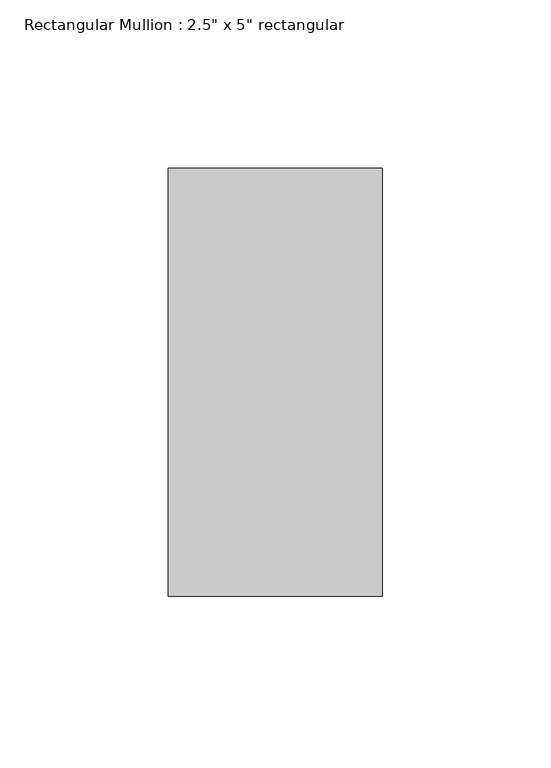
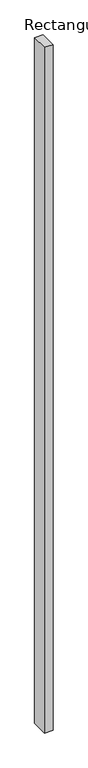
"""IFC4 building model written with IfcOpenShell, lengths in millimetres: member geometry."""

from ifc_helpers import new_model, si_unit, frame, origin, place, context, project, spatial, polyline, outline, extrude, source, transform, mapped, element, save


def member_753b68dd(model_context):
    return source(origin(), model_context, "Body", "SweptSolid", [
        extrude(outline(polyline([(0.0, 63.5), (0.0, -63.5), (-63.5, -63.5), (-63.5, 63.5), (0.0, 63.5)])), frame((0.0, 0.0, -5411.3315635), z_axis=(0.0, 0.0, 1.0), x_axis=(1.0, 0.0, 0.0)), (0.0, 0.0, 1.0), 5411.3315635),
    ])


if __name__ == "__main__":
    model = new_model("IFC4")
    model_context = context("Model", 3, world=origin())
    ifc_project = project(units=[si_unit("LENGTHUNIT", "METRE", prefix="MILLI")], contexts=[model_context])
    site = spatial("IfcSite", under=ifc_project)
    building = spatial("IfcBuilding", under=site)
    placement = place(None, origin())
    member_shape = member_753b68dd(model_context)
    element("IfcMember", 1, ObjectType="Rectangular Mullion : 2.5\" x 5\" rectangular", at=placement, inside=building, context=model_context, shape_type="MappedRepresentation", body=[
        mapped(member_shape, transform((0.0, 0.0, 0.0), x_axis=(1.0, 0.0, 0.0), y_axis=(0.0, 1.0, 0.0), z_axis=(0.0, 0.0, 1.0))),
    ])
    save(model, "model.ifc")

# Revit data of these elements
# Type "Rectangular Mullion : 2.5\" x 5\" rectangular"
#   built-in parameter 1007304 = 0.416667 (stored number, unit not read)
#   built-in parameter 1007301 = 0.104167 (stored number, unit not read)
#   built-in parameter 1007300 = 0.104167 (stored number, unit not read)
# Element 1 (IfcMember, "Rectangular Mullion : 2.5\" x 5\" rectangular")
#   Materials on its faces: "Aluminum"
# Materials
#   "Aluminum": class "Metal", colour RGB 247 247 247, transparency 0, Description = "Aluminum 6061", Cost = 0
